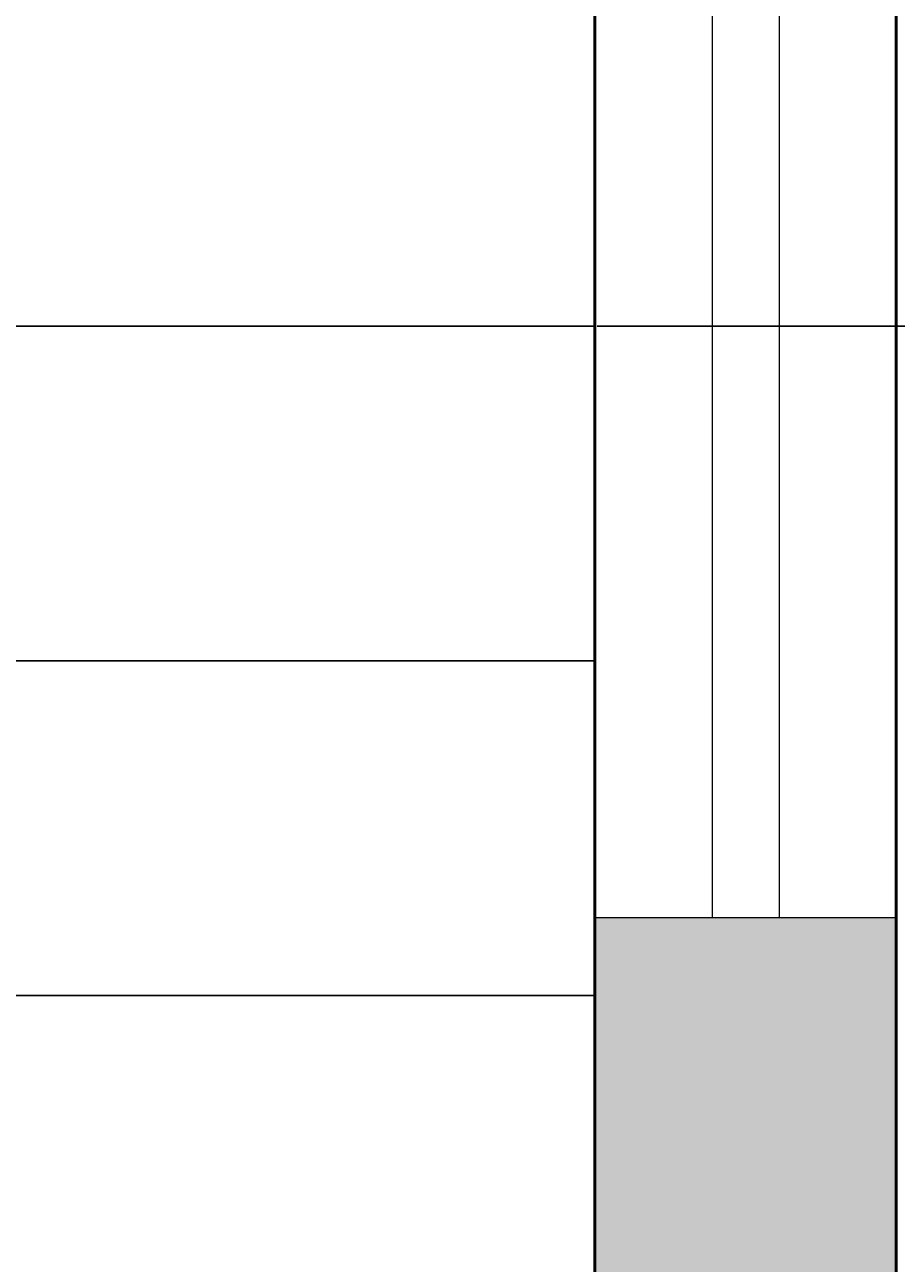
# Model space of a CAD drawing. Units: inches. Extents: x 2231 to 2461, y 2045 to 2455.
# Tile 65 of 95: x 2416 to 2442, y 2259 to 2296. Entities that reach past the tile are written whole.
import ezdxf

# ---------------------------------------------------------------- set-up
doc = ezdxf.new("R2010")
doc.units = ezdxf.units.IN
for name, color, linetype, lineweight in [('A-ANNO-DIMS', 2, 'Continuous', 18), ('A-FLOR-STRS', 7, 'Continuous', 25), ('A-GLAZ', 4, 'Continuous', 18), ('A-WALL', 7, 'Continuous', 50)]:
    doc.layers.add(name, color=color, linetype=linetype, lineweight=lineweight)
doc.layers.add('A-WALL-PATT', color=18, linetype='Continuous', lineweight=13, true_color=0x000000)
doc.styles.get("Standard").update_dxf_attribs({"font": 'arial.ttf'})
doc.dimstyles.get("Standard").update_dxf_attribs({"dimtxt": 0.18, "dimasz": 0.18, "dimexe": 0.18, "dimexo": 0.0625, "dimgap": 0.09, "dimtad": 0, "dimtih": 1, "dimtoh": 1, "dimdec": 4, "dimzin": 0, "dimdsep": 46, "dimtxsty": 'Standard', "dimcen": 0.09, "dimadec": 0, "dimazin": 0, "dimtfac": 1, "dimtdec": 4, "dimtofl": 0, "dimtmove": 0, "dimatfit": 3, "dimfxl": 1, "dimtolj": 1, "dimtzin": 0, "dimarcsym": 0})

# ---------------------------------------------------------------- blocks, each defined once
blk = doc.blocks.new('WIN-48IN')
for p, q in [((48, 9), (48, 0)), ((0, 5.5), (48, 5.5)), ((0, 3.5), (48, 3.5))]:
    blk.add_line(p, q)
blk = doc.blocks.new('*D42')
at = {"layer": 'A-ANNO-DIMS', "color": 0, "lineweight": -2, "transparency": 16777216}
for p, q in [((2396.794, 2286.895), (2396.794, 2454.645)), ((2432.794, 2286.895), (2432.794, 2454.645)), ((2396.974, 2454.465), (2414.575, 2454.465)), ((2432.614, 2454.465), (2415.012, 2454.465))]:
    blk.add_line(p, q, dxfattribs=at)
at = {"layer": 'A-ANNO-DIMS', "color": 0, "transparency": 16777216}
for points in [[(2396.974, 2454.495), (2396.974, 2454.435), (2396.794, 2454.465)], [(2432.614, 2454.495), (2432.614, 2454.435), (2432.794, 2454.465)]]:
    blk.add_solid(points, dxfattribs=at)
at = {"layer": 'Defpoints', "color": 0, "transparency": 16777216}
for p in [(2432.794, 2454.465), (2396.794, 2286.833), (2432.794, 2286.833)]:
    blk.add_point(p, dxfattribs=at)
at = {"layer": 'A-ANNO-DIMS', "color": 0, "transparency": 16777216, "insert": (2414.794, 2454.465), "char_height": 0.18, "attachment_point": 5}
blk.add_mtext('\\A1;36', dxfattribs=at)
blk = doc.blocks.new('*D43')
at = {"layer": 'A-ANNO-DIMS', "color": 0, "lineweight": -2, "transparency": 16777216}
for p, q in [((2432.856, 2286.833), (2460.606, 2286.833)), ((2460.426, 2286.653), (2460.426, 2237.015)), ((2460.426, 2187.013), (2460.426, 2236.651)), ((2432.856, 2186.833), (2460.606, 2186.833))]:
    blk.add_line(p, q, dxfattribs=at)
at = {"layer": 'A-ANNO-DIMS', "color": 0, "transparency": 16777216}
for points in [[(2460.396, 2286.653), (2460.456, 2286.653), (2460.426, 2286.833)], [(2460.396, 2187.013), (2460.456, 2187.013), (2460.426, 2186.833)]]:
    blk.add_solid(points, dxfattribs=at)
at = {"layer": 'Defpoints', "color": 0, "transparency": 16777216}
for p in [(2432.794, 2286.833), (2460.426, 2286.833), (2432.794, 2186.833)]:
    blk.add_point(p, dxfattribs=at)
at = {"layer": 'A-ANNO-DIMS', "color": 0, "transparency": 16777216, "insert": (2460.426, 2236.833), "char_height": 0.18, "attachment_point": 5}
blk.add_mtext('\\A1;100', dxfattribs=at)
blk = doc.blocks.new('*D59')
at = {"layer": 'A-ANNO-DIMS', "color": 0, "lineweight": -2, "transparency": 16777216}
for p, q in [((2408.794, 2182.895), (2408.794, 2454.645)), ((2432.794, 2182.895), (2432.794, 2454.645)), ((2408.974, 2454.465), (2420.573, 2454.465)), ((2432.614, 2454.465), (2421.014, 2454.465))]:
    blk.add_line(p, q, dxfattribs=at)
at = {"layer": 'A-ANNO-DIMS', "color": 0, "transparency": 16777216}
for points in [[(2408.974, 2454.495), (2408.974, 2454.435), (2408.794, 2454.465)], [(2432.614, 2454.495), (2432.614, 2454.435), (2432.794, 2454.465)]]:
    blk.add_solid(points, dxfattribs=at)
at = {"layer": 'Defpoints', "color": 0, "transparency": 16777216}
for p in [(2432.794, 2454.465), (2408.794, 2182.833), (2432.794, 2182.833)]:
    blk.add_point(p, dxfattribs=at)
at = {"layer": 'A-ANNO-DIMS', "color": 0, "transparency": 16777216, "insert": (2420.794, 2454.465), "char_height": 0.18, "attachment_point": 5}
blk.add_mtext('\\A1;24', dxfattribs=at)

msp = doc.modelspace()

# ---------------------------------------------------------------- hatches: boundary and pattern name
at = {"layer": 'A-WALL-PATT'}
h = msp.add_hatch(color=256, dxfattribs=at)
h.dxf.hatch_style = 1
h.paths.add_polyline_path([(2441.7935, 2269.1535), (2432.7935, 2269.1535), (2432.7935, 2186.8328), (2396.7935, 2186.8328), (2396.7935, 2286.8328), (2394.7935, 2286.8328), (2394.7935, 2186.8328), (2334.7935, 2186.8328), (2334.7935, 2182.8328), (2432.7935, 2182.8328), (2432.7935, 2072.8328), (2416.6639, 2072.8328), (2416.6639, 2063.8328), (2441.7935, 2063.8328)])
h.paths.add_polyline_path([(2368.6639, 2072.8328), (2367.04, 2072.8328), (2330.7942, 2072.8328), (2330.7397, 2063.8328), (2368.6639, 2063.8328)])
h.paths.add_polyline_path([(2300.7392, 2068.3328), (2300.7392, 2072.8328), (2298.7935, 2072.8328), (2294.7935, 2072.8328), (2258.7935, 2072.8328), (2258.7935, 2120.8328), (2294.7935, 2120.8328), (2298.7935, 2120.8328), (2298.7935, 2128.8328), (2294.7935, 2128.8328), (2294.7935, 2124.8328), (2258.7935, 2124.8328), (2258.7935, 2182.8328), (2294.7935, 2182.8328), (2294.7935, 2174.8328), (2298.7935, 2174.8328), (2298.7935, 2182.8328), (2304.7935, 2182.8328), (2304.7935, 2186.8328), (2258.7935, 2186.8328), (2258.7935, 2221.999), (2249.7935, 2221.999), (2249.7935, 2063.8328), (2300.7392, 2063.8328)])
h.paths.add_polyline_path([(2391.9338, 2435.8328), (2333.82, 2435.8328), (2333.82, 2426.8328), (2368.7935, 2426.8328), (2368.7935, 2374.9508), (2368.7935, 2370.8328), (2372.3935, 2370.8328), (2372.7935, 2370.8328), (2372.7935, 2426.8328), (2391.9338, 2426.8328)])
h.paths.add_polyline_path([(2441.7935, 2435.8328), (2415.9338, 2435.8328), (2415.9338, 2426.8328), (2432.7935, 2426.8328), (2432.7935, 2334.8328), (2372.7935, 2334.8328), (2372.7935, 2346.8328), (2368.7935, 2346.8328), (2368.7935, 2306.8328), (2360.7935, 2306.8328), (2360.7935, 2302.8328), (2368.7935, 2302.8328), (2372.7935, 2302.8328), (2372.7935, 2330.8328), (2432.7935, 2330.8328), (2432.7935, 2317.1535), (2441.7935, 2317.1535)])
h.paths.add_polyline_path([(2285.82, 2435.8328), (2249.7935, 2435.8328), (2249.7935, 2269.999), (2258.7935, 2269.999), (2258.7935, 2302.8328), (2318.8168, 2302.8328), (2330.7935, 2302.8328), (2330.7935, 2306.8328), (2258.7935, 2306.8328), (2258.7935, 2426.8328), (2285.82, 2426.8328)])

# ---------------------------------------------------------------- linework, layer by layer
at = {"layer": 'A-FLOR-STRS'}
for p, q in [((2394.7935, 2286.8328), (2432.7935, 2286.8328)), ((2396.7935, 2276.8328), (2432.7935, 2276.8328)), ((2396.7935, 2266.8328), (2432.7935, 2266.8328))]:
    msp.add_line(p, q, dxfattribs=at)
at = {"layer": 'A-WALL'}
msp.add_line((2432.7935, 2330.8328), (2432.7935, 2186.8328), dxfattribs=at)
msp.add_lwpolyline([(2300.7392, 2063.8328), (2249.7935, 2063.8328), (2249.7935, 2435.8328), (2441.7935, 2435.8328), (2441.7935, 2063.8328), (2330.7397, 2063.8328)], dxfattribs=at)

# ---------------------------------------------------------------- block references
at = {"layer": 'A-GLAZ', "rotation": 270.0000000000023}
msp.add_blockref('WIN-48IN', (2432.7937, 2317.1535), dxfattribs=at)

# ---------------------------------------------------------------- dimensions: what is measured, and where the dimension line sits
at = {"layer": 'A-ANNO-DIMS'}
for p1, p2, picture, middle in [((2396.7935, 2286.8328), (2432.7935, 2286.8328), '*D42', (2414.7935, 2454.4653)), ((2408.7935, 2182.8328), (2432.7935, 2182.8328), '*D59', (2420.7935, 2454.4653))]:
    dim = msp.add_linear_dim(base=(2432.7935, 2454.4653), p1=p1, p2=p2, dimstyle='Standard', override={"dimdec": 0, "dimlfac": 1, "dimrnd": 0, "dimzin": 0, "dimdsep": 46, "dimlunit": 2}, dxfattribs=at)
    dim.commit()
    dim.dimension.update_dxf_attribs({"geometry": picture, "text_midpoint": middle})
dim = msp.add_linear_dim(base=(2460.426, 2286.8328), p1=(2432.7935, 2186.8328), p2=(2432.7935, 2286.8328), angle=90, dimstyle='Standard', override={"dimdec": 0, "dimlfac": 1, "dimrnd": 0, "dimzin": 0, "dimdsep": 46, "dimlunit": 2}, dxfattribs=at)
dim.commit()
dim.dimension.update_dxf_attribs({"geometry": '*D43', "text_midpoint": (2460.426, 2236.8328)})

doc.saveas('drawing.dxf')
